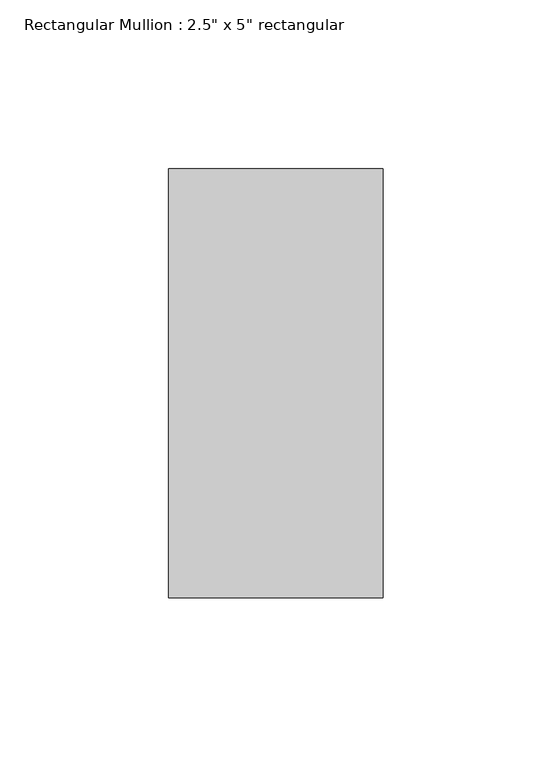
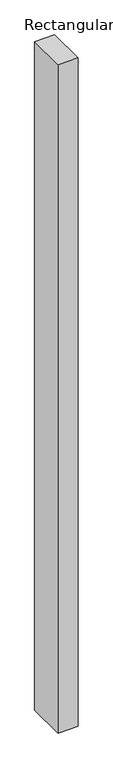
"""IFC4 building model written with IfcOpenShell, lengths in millimetres: member geometry."""

from ifc_helpers import new_model, si_unit, frame, origin, place, context, project, spatial, polyline, outline, extrude, source, transform, mapped, element, save


def member_4d8d05fd(model_context):
    return source(origin(), model_context, "Body", "SweptSolid", [
        extrude(outline(polyline([(31.75, 63.5), (31.75, -63.5), (-31.75, -63.5), (-31.75, 63.5), (31.75, 63.5)])), frame((0.0, 0.0, -2234.5154028), z_axis=(0.0, 0.0, 1.0), x_axis=(1.0, 0.0, 0.0)), (0.0, 0.0, 1.0), 2234.5154028),
    ])


if __name__ == "__main__":
    model = new_model("IFC4")
    model_context = context("Model", 3, world=origin())
    ifc_project = project(units=[si_unit("LENGTHUNIT", "METRE", prefix="MILLI")], contexts=[model_context])
    site = spatial("IfcSite", under=ifc_project)
    building = spatial("IfcBuilding", under=site)
    placement = place(None, origin())
    member_shape = member_4d8d05fd(model_context)
    element("IfcMember", 1, ObjectType="Rectangular Mullion : 2.5\" x 5\" rectangular", at=placement, inside=building, context=model_context, shape_type="MappedRepresentation", body=[
        mapped(member_shape, transform((0.0, 0.0, 0.0), x_axis=(1.0, 0.0, 0.0), y_axis=(0.0, 1.0, 0.0), z_axis=(0.0, 0.0, 1.0))),
    ])
    save(model, "model.ifc")

# Revit data of these elements
# Type "Rectangular Mullion : 2.5\" x 5\" rectangular"
#   built-in parameter 1007304 = 0.416667 (stored number, unit not read)
#   built-in parameter 1007301 = 0.104167 (stored number, unit not read)
#   built-in parameter 1007300 = 0.104167 (stored number, unit not read)
# Element 1 (IfcMember, "Rectangular Mullion : 2.5\" x 5\" rectangular")
#   Materials on its faces: "Aluminum"
# Materials
#   "Aluminum": class "Metal", colour RGB 247 247 247, transparency 0, Description = "Aluminum 6061", Cost = 0
